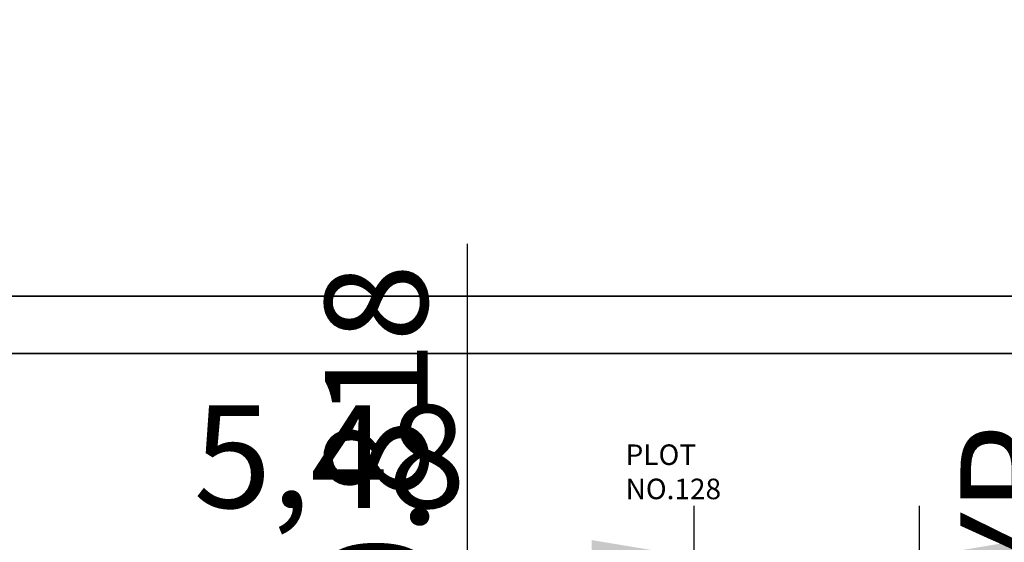
# Model space of a CAD drawing. Units: metres. Extents: x 782 to 1487, y 1262 to 7446.
# Tile 23 of 25: x 802 to 826, y 1337 to 1350. Entities that reach past the tile are written whole.
import ezdxf

# ---------------------------------------------------------------- set-up
doc = ezdxf.new("R2010")
doc.units = ezdxf.units.M
for name, color, linetype, lineweight in [('A-ANNO-DIMS', 2, 'Continuous', 18), ('A-ANNO-TEXT', 3, 'Continuous', 18), ('A-ANNO-TTLB', 7, 'Continuous', 35)]:
    doc.layers.add(name, color=color, linetype=linetype, lineweight=lineweight)
doc.styles.get("Standard").update_dxf_attribs({"font": 'arial.ttf'})
doc.dimstyles.new('ISO-25', dxfattribs={"dimtxt": 2.5, "dimasz": 2.5, "dimexe": 1.25, "dimexo": 0.625, "dimtad": 1, "dimtxsty": 'Standard', "dimcen": 2.5, "dimadec": 0, "dimazin": 0, "dimtfac": 1, "dimtmove": 0, "dimatfit": 3, "dimfxl": 1, "dimarcsym": 0})

# ---------------------------------------------------------------- blocks, each defined once
blk = doc.blocks.new('*D12')
at = {"layer": 'A-ANNO-DIMS', "color": 0, "lineweight": -2, "transparency": 16777216}
for p, q in [((818.357, 1335.252), (818.357, 1337.877)), ((823.837, 1335.252), (823.837, 1337.877)), ((815.857, 1336.627), (805.608, 1336.627)), ((823.837, 1336.627), (818.357, 1336.627)), ((826.337, 1336.627), (828.837, 1336.627))]:
    blk.add_line(p, q, dxfattribs=at)
at = {"layer": 'A-ANNO-DIMS', "color": 0, "transparency": 16777216}
for points in [[(815.857, 1337.044), (815.857, 1336.21), (818.357, 1336.627)], [(826.337, 1337.044), (826.337, 1336.21), (823.837, 1336.627)]]:
    blk.add_solid(points, dxfattribs=at)
at = {"layer": 'Defpoints', "color": 0, "transparency": 16777216}
for p in [(818.357, 1336.627), (818.357, 1334.627), (823.837, 1334.627)]:
    blk.add_point(p, dxfattribs=at)
at = {"layer": 'A-ANNO-DIMS', "color": 0, "transparency": 16777216, "insert": (809.482, 1338.754), "char_height": 2.5, "width": 6.51678, "attachment_point": 5}
blk.add_mtext('5,48', dxfattribs=at)
blk = doc.blocks.new('*D20')
at = {"layer": 'A-ANNO-DIMS', "color": 0, "lineweight": -2, "transparency": 16777216}
for p, q in [((831.056, 1302.088), (831.056, 1337.678)), ((831.056, 1298.698), (831.056, 1299.588)), ((831.548, 1299.588), (832.306, 1299.588)), ((831.548, 1298.698), (832.306, 1298.698)), ((831.056, 1296.198), (831.056, 1293.698))]:
    blk.add_line(p, q, dxfattribs=at)
at = {"layer": 'A-ANNO-DIMS', "color": 0, "transparency": 16777216}
for points in [[(830.64, 1302.088), (831.473, 1302.088), (831.056, 1299.588)], [(830.64, 1296.198), (831.473, 1296.198), (831.056, 1298.698)]]:
    blk.add_solid(points, dxfattribs=at)
at = {"layer": 'Defpoints', "color": 0, "transparency": 16777216}
for p in [(830.923, 1299.588), (831.056, 1299.588), (830.923, 1298.698)]:
    blk.add_point(p, dxfattribs=at)
at = {"layer": 'A-ANNO-DIMS', "color": 0, "transparency": 16777216, "insert": (829.138, 1321.133), "char_height": 2.5, "attachment_point": 5, "rotation": 90}
blk.add_mtext('DOOR D1 0.89 TYP.', dxfattribs=at)
blk = doc.blocks.new('*D26')
at = {"layer": 'A-ANNO-DIMS', "color": 0, "lineweight": -2, "transparency": 16777216}
for p, q in [((828.33, 1303.223), (828.33, 1342.718)), ((828.33, 1299.809), (828.33, 1300.723)), ((828.818, 1300.723), (829.58, 1300.723)), ((828.818, 1299.809), (829.58, 1299.809)), ((828.33, 1297.309), (828.33, 1294.809))]:
    blk.add_line(p, q, dxfattribs=at)
at = {"layer": 'A-ANNO-DIMS', "color": 0, "transparency": 16777216}
for points in [[(827.913, 1303.223), (828.747, 1303.223), (828.33, 1300.723)], [(827.913, 1297.309), (828.747, 1297.309), (828.33, 1299.809)]]:
    blk.add_solid(points, dxfattribs=at)
at = {"layer": 'Defpoints', "color": 0, "transparency": 16777216}
for p in [(828.193, 1300.723), (828.33, 1300.723), (828.193, 1299.809)]:
    blk.add_point(p, dxfattribs=at)
at = {"layer": 'A-ANNO-DIMS', "color": 0, "transparency": 16777216, "insert": (826.412, 1324.22), "char_height": 2.5, "attachment_point": 5, "rotation": 90}
blk.add_mtext('WINDOW W 0.91 TYP.', dxfattribs=at)
blk = doc.blocks.new('*D28')
at = {"layer": 'A-ANNO-DIMS', "color": 0, "lineweight": -2, "transparency": 16777216}
for p, q in [((832.55, 1308.281), (832.55, 1349.718)), ((832.55, 1304.867), (832.55, 1305.781)), ((833.038, 1305.781), (833.8, 1305.781)), ((833.038, 1304.867), (833.8, 1304.867)), ((832.55, 1302.367), (832.55, 1299.867))]:
    blk.add_line(p, q, dxfattribs=at)
at = {"layer": 'A-ANNO-DIMS', "color": 0, "transparency": 16777216}
for points in [[(832.134, 1308.281), (832.967, 1308.281), (832.55, 1305.781)], [(832.134, 1302.367), (832.967, 1302.367), (832.55, 1304.867)]]:
    blk.add_solid(points, dxfattribs=at)
at = {"layer": 'Defpoints', "color": 0, "transparency": 16777216}
for p in [(832.413, 1305.781), (832.55, 1305.781), (832.413, 1304.867)]:
    blk.add_point(p, dxfattribs=at)
at = {"layer": 'A-ANNO-DIMS', "color": 0, "transparency": 16777216, "insert": (830.632, 1330.25), "char_height": 2.5, "attachment_point": 5, "rotation": 90}
blk.add_mtext('WINDOW W1 0.91 TYP.', dxfattribs=at)
blk = doc.blocks.new('*D146')
at = {"layer": 'A-ANNO-DIMS', "color": 0, "lineweight": -2, "transparency": 16777216}
for p, q in [((812.839, 1330.363), (812.839, 1344.262)), ((810.513, 1330.363), (814.089, 1330.363)), ((812.839, 1322.045), (812.839, 1327.863)), ((810.513, 1319.545), (814.089, 1319.545))]:
    blk.add_line(p, q, dxfattribs=at)
at = {"layer": 'A-ANNO-DIMS', "color": 0, "transparency": 16777216}
for points in [[(812.422, 1327.863), (813.255, 1327.863), (812.839, 1330.363)], [(812.422, 1322.045), (813.255, 1322.045), (812.839, 1319.545)]]:
    blk.add_solid(points, dxfattribs=at)
at = {"layer": 'Defpoints', "color": 0, "transparency": 16777216}
for p in [(809.888, 1330.363), (812.839, 1330.363), (809.888, 1319.545)]:
    blk.add_point(p, dxfattribs=at)
at = {"layer": 'A-ANNO-DIMS', "color": 0, "transparency": 16777216, "insert": (810.937, 1338.563), "char_height": 2.5, "attachment_point": 5, "rotation": 90}
blk.add_mtext('10.818', dxfattribs=at)

msp = doc.modelspace()

# ---------------------------------------------------------------- linework, layer by layer
at = {"layer": 'A-ANNO-TTLB'}
for points in [[(787.4248, 1342.9861), (880.8003, 1342.9861), (880.8003, 1263.8004), (787.4248, 1263.8004)], [(883.6865, 1262.3458), (787.4248, 1262.3458), (787.4248, 1342.9861), (883.6865, 1342.9861)], [(788.8147, 1341.5907), (880.8003, 1341.5907), (880.8003, 1263.8004), (788.8147, 1263.8004)]]:
    msp.add_lwpolyline(points, close=True, dxfattribs=at)

# ---------------------------------------------------------------- texts
at = {"layer": 'A-ANNO-TEXT', "insert": (816.6847, 1339.3731), "char_height": 0.5, "attachment_point": 1}
msp.add_mtext_dynamic_manual_height_columns('PLOT NO.128', width=3.78564, gutter_width=12.5, heights=[0], dxfattribs=at)

# ---------------------------------------------------------------- dimensions: what is measured, and where the dimension line sits
at = {"layer": 'A-ANNO-DIMS'}
for base, p1, p2, text, picture, middle in [((832.5503, 1305.7809), (832.4132, 1304.8669), (832.4132, 1305.7809), 'WINDOW W1 <> TYP.', '*D28', (830.6318, 1330.2497)), ((828.3302, 1300.7228), (828.1931, 1299.8088), (828.1931, 1300.7228), 'WINDOW W <> TYP.', '*D26', (826.4117, 1324.2204)), ((831.0564, 1299.5877), (830.923, 1298.6982), (830.923, 1299.5877), 'DOOR D1 <> TYP.', '*D20', (829.138, 1321.1327))]:
    dim = msp.add_linear_dim(base=base, p1=p1, p2=p2, angle=90, text=text, dimstyle='ISO-25', override={"dimdec": 2, "dimlfac": 1, "dimrnd": 0, "dimzin": 0, "dimdsep": 46, "dimlunit": 2}, dxfattribs=at)
    dim.commit()
    dim.dimension.update_dxf_attribs({"geometry": picture, "text_midpoint": middle})
dim = msp.add_linear_dim(base=(812.8387, 1330.3635), p1=(809.8881, 1319.5451), p2=(809.8881, 1330.3635), angle=90, dimstyle='ISO-25', override={"dimdec": 3, "dimlfac": 1, "dimrnd": 0, "dimzin": 0, "dimdsep": 46, "dimlunit": 2}, dxfattribs=at)
dim.commit()
dim.dimension.update_dxf_attribs({"geometry": '*D146', "text_midpoint": (810.9373, 1338.5627)})
dim = msp.add_linear_dim(base=(818.357, 1336.627), p1=(823.837, 1334.627), p2=(818.357, 1334.627), dimstyle='ISO-25', override={"dimclrd": 0, "dimclre": 0, "dimclrt": 0}, dxfattribs=at)
dim.commit()
dim.dimension.update_dxf_attribs({"geometry": '*D12', "text_midpoint": (809.4825, 1338.7544)})

doc.saveas('drawing.dxf')
